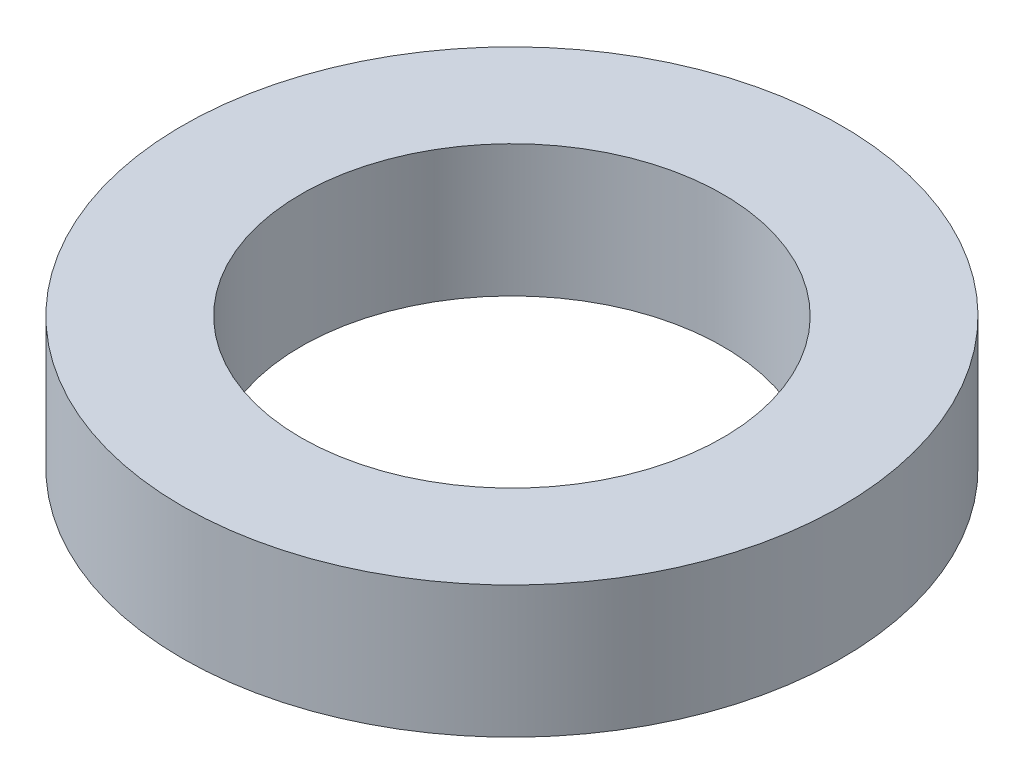
from build123d import *

# Parameters (mm, degrees)
WASHER_PROFILE_50_32_R   = 25
WASHER_PROFILE_50_32_R_2 = 16
WASHER_BODY_10MM_DEPTH   = 10


with BuildPart() as part:
    # Washer Profile Ø50-Ø32 → Washer Body 10mm (new body)
    with BuildSketch(Plane(origin=(0, 0, 0), x_dir=(1, 0, 0), z_dir=(0, 1, 0))):
        with Locations(Location((0, 0, 0), (0, 0, 270))):
            Circle(WASHER_PROFILE_50_32_R)
        with Locations(Location((0, 0, 0), (0, 0, 270))):
            Circle(WASHER_PROFILE_50_32_R_2, mode=Mode.SUBTRACT)
    extrude(amount=WASHER_BODY_10MM_DEPTH)


solid = part.part
